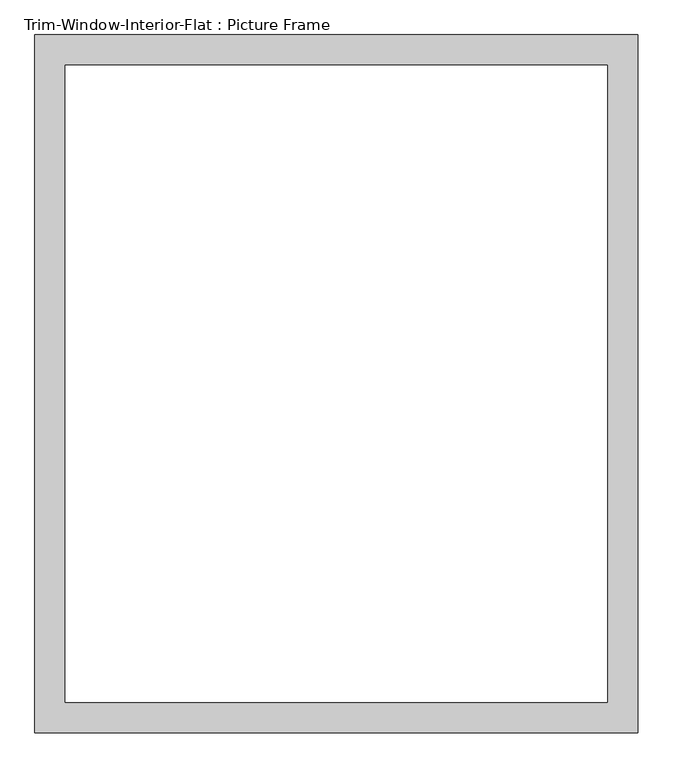
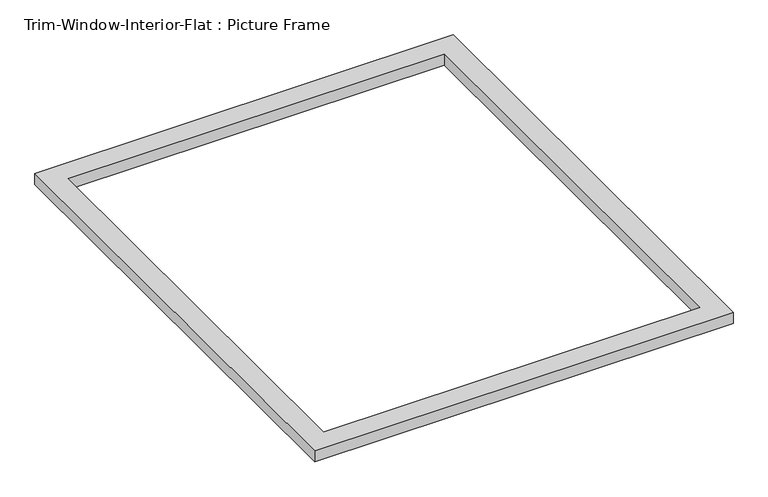
"""IFC4 building model written with IfcOpenShell, lengths in millimetres: proxy geometry, Trim-Window-Interior-Flat : Picture Frame."""

from ifc_helpers import new_model, si_unit, origin, origin_with_axes, place, context, project, spatial, polyline, outline, extrude, source, transform, mapped, element, save


def trim_window_interior_flat_picture_frame_56711e78(model_context):
    return source(origin(), model_context, "Body", "SweptSolid", [
        extrude(outline(polyline([(565.15, 44.45), (565.15, -1263.65), (-565.15, -1263.65), (-565.15, 44.45), (565.15, 44.45)]), holes=[polyline([(508.0, -12.7), (-508.0, -12.7), (-508.0, -1206.5), (508.0, -1206.5), (508.0, -12.7)])]), origin_with_axes(), (0.0, 0.0, 1.0), 31.75),
    ])


if __name__ == "__main__":
    model = new_model("IFC4")
    model_context = context("Model", 3, world=origin())
    ifc_project = project(units=[si_unit("LENGTHUNIT", "METRE", prefix="MILLI")], contexts=[model_context])
    site = spatial("IfcSite", under=ifc_project)
    building = spatial("IfcBuilding", under=site)
    placement = place(None, origin())
    trim_window_interior_flat_picture_frame_shape = trim_window_interior_flat_picture_frame_56711e78(model_context)
    element("IfcBuildingElementProxy", 1, Name="Trim-Window-Interior-Flat : Picture Frame", ObjectType="Trim-Window-Interior-Flat : Picture Frame", at=placement, inside=building, context=model_context, shape_type="MappedRepresentation", body=[
        mapped(trim_window_interior_flat_picture_frame_shape, transform((0.0, 0.0, 0.0), x_axis=(1.0, 0.0, 0.0), y_axis=(0.0, 1.0, 0.0), z_axis=(0.0, 0.0, 1.0))),
    ])
    save(model, "model.ifc")

# Revit data of these elements
# Type "Trim-Window-Interior-Flat : Picture Frame"
#   Trim Thickness_Picture Frame = 0' - 1 1/4"
#   Trim Width = 0' - 2 1/4"
#   Trim Thickness_with Sill = 0' - 0 3/4"
#   Sill Thickness = 0' - 1 1/4"
#   Opening Width [instance default] = 2' - 0"
#   Opening Height [instance default] = 3' - 0"
#   Default Elevation = 4' - 0"
#   Sill = no
#   Picture Frame = yes
#   Trim Material [instance default] = none
# Element 1 (IfcBuildingElementProxy, "Trim-Window-Interior-Flat : Picture Frame")
#   Opening Width = 3' - 5"
#   Opening Height = 4' - 0"
#   Trim Material = Wood - Stained
#   Materials on its faces: "Wood - Stained"
# Materials
#   "Wood - Stained": class "Wood", colour RGB 224 178 126, transparency 0, Cost = 0
